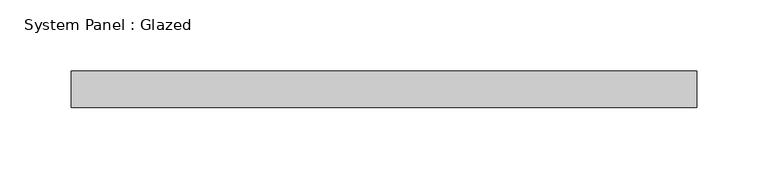
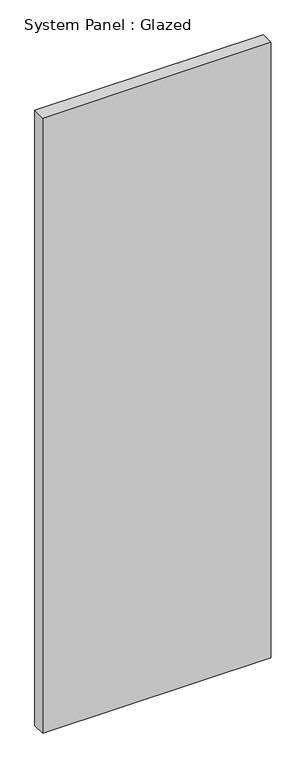
"""IFC4 building model written with IfcOpenShell, lengths in millimetres: plate geometry, System Panel : Glazed."""

from ifc_helpers import new_model, si_unit, origin, origin_with_axes, place, context, project, spatial, polyline, outline, extrude, source, transform, mapped, element, save


def system_panel_glazed_f327d843(model_context):
    return source(origin(), model_context, "Body", "SweptSolid", [
        extrude(outline(polyline([(219.075, 19.05), (-219.075, 19.05), (-219.075, 44.45), (219.075, 44.45), (219.075, 19.05)])), origin_with_axes(), (0.0, 0.0, 1.0), 1248.9446538),
    ])


if __name__ == "__main__":
    model = new_model("IFC4")
    model_context = context("Model", 3, world=origin())
    ifc_project = project(units=[si_unit("LENGTHUNIT", "METRE", prefix="MILLI")], contexts=[model_context])
    site = spatial("IfcSite", under=ifc_project)
    building = spatial("IfcBuilding", under=site)
    placement = place(None, origin())
    system_panel_glazed_shape = system_panel_glazed_f327d843(model_context)
    element("IfcPlate", 1, ObjectType="System Panel : Glazed", at=placement, inside=building, context=model_context, shape_type="MappedRepresentation", body=[
        mapped(system_panel_glazed_shape, transform((0.0, 0.0, 0.0), x_axis=(1.0, 0.0, 0.0), y_axis=(0.0, 1.0, 0.0), z_axis=(0.0, 0.0, 1.0))),
    ])
    save(model, "model.ifc")

# Revit data of these elements
# Type "System Panel : Glazed"
#   Construction Type Id = "GSP4R"
#   Analytic Construction = "1/8 in Pilkington single glazing"
#   Visual Light Transmittance = 0.9
#   Solar Heat Gain Coefficient = 0.86
#   Heat Transfer Coefficient (U) = 1.18115 BTU/(h·ft²·°F)
#   Define Thermal Properties by = 1
# Element 1 (IfcPlate, "System Panel : Glazed")
#   Materials on its faces: "Glass"
# Materials
#   "Glass": class "Glass", colour RGB 0 128 192, transparency 0.75, Description = "Soda Lime Glass", Cost = 0
